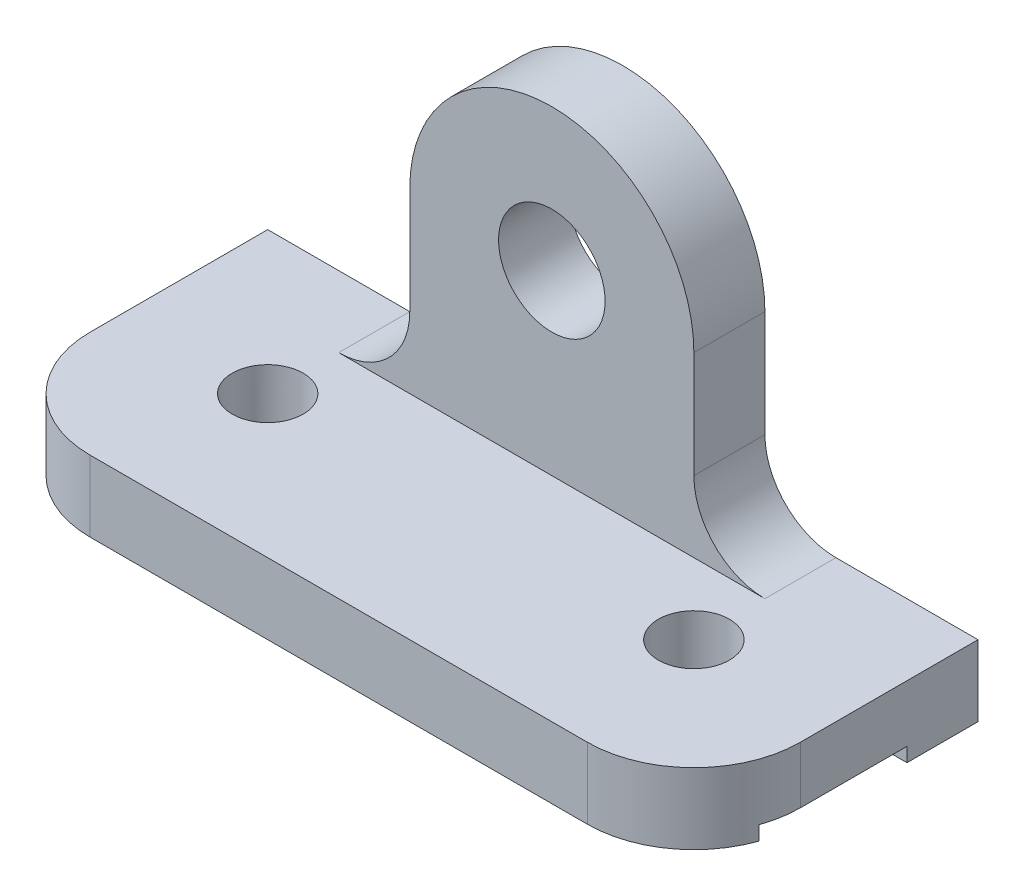
ISO-10303-21;
HEADER;
FILE_DESCRIPTION(('STEP AP214'),'2;1');
FILE_NAME('part.step','',(''),(''),'','','');
FILE_SCHEMA(('AUTOMOTIVE_DESIGN { 1 0 10303 214 1 1 1 1 }'));
ENDSEC;
DATA;
#1=APPLICATION_CONTEXT('core data for automotive mechanical design processes');
#2=APPLICATION_PROTOCOL_DEFINITION('international standard','automotive_design',2000,#1);
#3=PRODUCT_CONTEXT('',#1,'mechanical');
#4=PRODUCT('Part','Part','',(#3));
#5=PRODUCT_RELATED_PRODUCT_CATEGORY('part','',(#4));
#6=PRODUCT_DEFINITION_FORMATION('','',#4);
#7=PRODUCT_DEFINITION_CONTEXT('part definition',#1,'design');
#8=PRODUCT_DEFINITION('design','',#6,#7);
#9=PRODUCT_DEFINITION_SHAPE('','',#8);
#10=(LENGTH_UNIT() NAMED_UNIT(*) SI_UNIT(.MILLI.,.METRE.));
#11=(NAMED_UNIT(*) PLANE_ANGLE_UNIT() SI_UNIT($,.RADIAN.));
#12=(NAMED_UNIT(*) SI_UNIT($,.STERADIAN.) SOLID_ANGLE_UNIT());
#13=UNCERTAINTY_MEASURE_WITH_UNIT(LENGTH_MEASURE(1.E-05),#10,'distance_accuracy_value','');
#14=(GEOMETRIC_REPRESENTATION_CONTEXT(3) GLOBAL_UNCERTAINTY_ASSIGNED_CONTEXT((#13)) GLOBAL_UNIT_ASSIGNED_CONTEXT((#10,
#11,#12)) REPRESENTATION_CONTEXT('',''));
#15=CARTESIAN_POINT('',(0.,0.,0.));
#16=DIRECTION('',(0.,0.,1.));
#17=DIRECTION('',(1.,0.,0.));
#18=AXIS2_PLACEMENT_3D('',#15,#16,#17);
#19=CARTESIAN_POINT('',(-50.,0.,40.));
#20=DIRECTION('',(-1.,0.,0.));
#21=DIRECTION('',(0.,0.,1.));
#22=AXIS2_PLACEMENT_3D('',#19,#20,#21);
#23=PLANE('',#22);
#24=DIRECTION('',(0.,1.,0.));
#25=VECTOR('',#24,1.);
#26=CARTESIAN_POINT('',(-50.,0.,10.));
#27=LINE('',#26,#25);
#28=CARTESIAN_POINT('',(-50.,0.,10.));
#29=VERTEX_POINT('',#28);
#30=CARTESIAN_POINT('',(-50.,2.00000000000002,10.));
#31=VERTEX_POINT('',#30);
#32=EDGE_CURVE('E165',#29,#31,#27,.T.);
#33=ORIENTED_EDGE('',*,*,#32,.T.);
#34=DIRECTION('',(0.,0.,1.));
#35=VECTOR('',#34,1.);
#36=CARTESIAN_POINT('',(-50.,2.00000000000002,30.));
#37=LINE('',#36,#35);
#38=CARTESIAN_POINT('',(-50.,2.00000000000002,25.));
#39=VERTEX_POINT('',#38);
#40=EDGE_CURVE('E234',#31,#39,#37,.T.);
#41=ORIENTED_EDGE('',*,*,#40,.T.);
#42=DIRECTION('',(0.,1.,0.));
#43=VECTOR('',#42,1.);
#44=CARTESIAN_POINT('',(-50.,0.,25.));
#45=LINE('',#44,#43);
#46=CARTESIAN_POINT('',(-50.,10.,25.));
#47=VERTEX_POINT('',#46);
#48=EDGE_CURVE('E220',#39,#47,#45,.T.);
#49=ORIENTED_EDGE('',*,*,#48,.T.);
#50=DIRECTION('',(0.,0.,-1.));
#51=VECTOR('',#50,1.);
#52=CARTESIAN_POINT('',(-50.,10.,40.));
#53=LINE('',#52,#51);
#54=CARTESIAN_POINT('',(-50.,10.,0.));
#55=VERTEX_POINT('',#54);
#56=EDGE_CURVE('E184',#47,#55,#53,.T.);
#57=ORIENTED_EDGE('',*,*,#56,.T.);
#58=DIRECTION('',(0.,1.,0.));
#59=VECTOR('',#58,1.);
#60=CARTESIAN_POINT('',(-50.,0.,0.));
#61=LINE('',#60,#59);
#62=CARTESIAN_POINT('',(-50.,0.,0.));
#63=VERTEX_POINT('',#62);
#64=EDGE_CURVE('E254',#63,#55,#61,.T.);
#65=ORIENTED_EDGE('',*,*,#64,.F.);
#66=DIRECTION('',(0.,0.,-1.));
#67=VECTOR('',#66,1.);
#68=CARTESIAN_POINT('',(-50.,0.,40.));
#69=LINE('',#68,#67);
#70=EDGE_CURVE('E182',#29,#63,#69,.T.);
#71=ORIENTED_EDGE('',*,*,#70,.F.);
#72=EDGE_LOOP('',(#33,#41,#49,#57,#65,#71));
#73=FACE_BOUND('',#72,.T.);
#74=ADVANCED_FACE('F43',(#73),#23,.T.);
#75=CARTESIAN_POINT('',(0.,0.,40.));
#76=DIRECTION('',(0.,1.,0.));
#77=DIRECTION('',(-1.,0.,0.));
#78=AXIS2_PLACEMENT_3D('',#75,#76,#77);
#79=PLANE('',#78);
#80=DIRECTION('',(1.,0.,0.));
#81=VECTOR('',#80,1.);
#82=CARTESIAN_POINT('',(-50.,0.,10.));
#83=LINE('',#82,#81);
#84=CARTESIAN_POINT('',(50.,0.,10.));
#85=VERTEX_POINT('',#84);
#86=EDGE_CURVE('E156',#29,#85,#83,.T.);
#87=ORIENTED_EDGE('',*,*,#86,.F.);
#88=ORIENTED_EDGE('',*,*,#70,.T.);
#89=DIRECTION('',(1.,0.,0.));
#90=VECTOR('',#89,1.);
#91=CARTESIAN_POINT('',(0.,0.,0.));
#92=LINE('',#91,#90);
#93=CARTESIAN_POINT('',(50.,0.,0.));
#94=VERTEX_POINT('',#93);
#95=EDGE_CURVE('E178',#63,#94,#92,.T.);
#96=ORIENTED_EDGE('',*,*,#95,.T.);
#97=DIRECTION('',(0.,0.,-1.));
#98=VECTOR('',#97,1.);
#99=CARTESIAN_POINT('',(50.,0.,40.));
#100=LINE('',#99,#98);
#101=EDGE_CURVE('E172',#85,#94,#100,.T.);
#102=ORIENTED_EDGE('',*,*,#101,.F.);
#103=EDGE_LOOP('',(#87,#88,#96,#102));
#104=FACE_BOUND('',#103,.T.);
#105=ADVANCED_FACE('F180',(#104),#79,.F.);
#106=CARTESIAN_POINT('',(50.,0.,40.));
#107=DIRECTION('',(1.,0.,0.));
#108=DIRECTION('',(0.,0.,-1.));
#109=AXIS2_PLACEMENT_3D('',#106,#107,#108);
#110=PLANE('',#109);
#111=DIRECTION('',(0.,1.,0.));
#112=VECTOR('',#111,1.);
#113=CARTESIAN_POINT('',(50.,0.,10.));
#114=LINE('',#113,#112);
#115=CARTESIAN_POINT('',(50.,2.00000000000002,10.));
#116=VERTEX_POINT('',#115);
#117=EDGE_CURVE('E157',#85,#116,#114,.T.);
#118=ORIENTED_EDGE('',*,*,#117,.F.);
#119=ORIENTED_EDGE('',*,*,#101,.T.);
#120=DIRECTION('',(0.,-1.,0.));
#121=VECTOR('',#120,1.);
#122=CARTESIAN_POINT('',(50.,0.,0.));
#123=LINE('',#122,#121);
#124=CARTESIAN_POINT('',(50.,10.,0.));
#125=VERTEX_POINT('',#124);
#126=EDGE_CURVE('E257',#125,#94,#123,.T.);
#127=ORIENTED_EDGE('',*,*,#126,.F.);
#128=DIRECTION('',(0.,0.,-1.));
#129=VECTOR('',#128,1.);
#130=CARTESIAN_POINT('',(50.,10.,40.));
#131=LINE('',#130,#129);
#132=CARTESIAN_POINT('',(50.,10.,25.));
#133=VERTEX_POINT('',#132);
#134=EDGE_CURVE('E192',#133,#125,#131,.T.);
#135=ORIENTED_EDGE('',*,*,#134,.F.);
#136=DIRECTION('',(0.,-1.,0.));
#137=VECTOR('',#136,1.);
#138=CARTESIAN_POINT('',(50.,0.,25.));
#139=LINE('',#138,#137);
#140=CARTESIAN_POINT('',(50.,2.00000000000002,25.));
#141=VERTEX_POINT('',#140);
#142=EDGE_CURVE('E198',#133,#141,#139,.T.);
#143=ORIENTED_EDGE('',*,*,#142,.T.);
#144=DIRECTION('',(0.,0.,1.));
#145=VECTOR('',#144,1.);
#146=CARTESIAN_POINT('',(50.,2.00000000000002,30.));
#147=LINE('',#146,#145);
#148=EDGE_CURVE('E175',#116,#141,#147,.T.);
#149=ORIENTED_EDGE('',*,*,#148,.F.);
#150=EDGE_LOOP('',(#118,#119,#127,#135,#143,#149));
#151=FACE_BOUND('',#150,.T.);
#152=ADVANCED_FACE('F168',(#151),#110,.T.);
#153=CARTESIAN_POINT('',(0.,10.,40.));
#154=DIRECTION('',(0.,1.,0.));
#155=DIRECTION('',(-1.,0.,0.));
#156=AXIS2_PLACEMENT_3D('',#153,#154,#155);
#157=PLANE('',#156);
#158=CARTESIAN_POINT('',(30.,10.,20.));
#159=DIRECTION('',(0.,1.,0.));
#160=DIRECTION('',(-1.,0.,0.));
#161=AXIS2_PLACEMENT_3D('',#158,#159,#160);
#162=CIRCLE('',#161,5.);
#163=CARTESIAN_POINT('',(25.,10.,20.));
#164=VERTEX_POINT('',#163);
#165=EDGE_CURVE('E281',#164,#164,#162,.F.);
#166=ORIENTED_EDGE('',*,*,#165,.T.);
#167=EDGE_LOOP('',(#166));
#168=FACE_BOUND('',#167,.T.);
#169=CARTESIAN_POINT('',(-30.,10.,20.));
#170=DIRECTION('',(0.,1.,0.));
#171=DIRECTION('',(-1.,0.,0.));
#172=AXIS2_PLACEMENT_3D('',#169,#170,#171);
#173=CIRCLE('',#172,5.);
#174=CARTESIAN_POINT('',(-35.,10.,20.));
#175=VERTEX_POINT('',#174);
#176=EDGE_CURVE('E294',#175,#175,#173,.F.);
#177=ORIENTED_EDGE('',*,*,#176,.T.);
#178=EDGE_LOOP('',(#177));
#179=FACE_BOUND('',#178,.T.);
#180=DIRECTION('',(1.,0.,0.));
#181=VECTOR('',#180,1.);
#182=CARTESIAN_POINT('',(0.,10.,40.));
#183=LINE('',#182,#181);
#184=CARTESIAN_POINT('',(-35.,10.,40.));
#185=VERTEX_POINT('',#184);
#186=CARTESIAN_POINT('',(35.,10.,40.));
#187=VERTEX_POINT('',#186);
#188=EDGE_CURVE('E187',#185,#187,#183,.T.);
#189=ORIENTED_EDGE('',*,*,#188,.T.);
#190=CARTESIAN_POINT('',(35.,10.,25.));
#191=DIRECTION('',(0.,1.,0.));
#192=DIRECTION('',(-1.,0.,0.));
#193=AXIS2_PLACEMENT_3D('',#190,#191,#192);
#194=CIRCLE('',#193,15.);
#195=EDGE_CURVE('E214',#187,#133,#194,.T.);
#196=ORIENTED_EDGE('',*,*,#195,.T.);
#197=ORIENTED_EDGE('',*,*,#134,.T.);
#198=DIRECTION('',(1.,0.,0.));
#199=VECTOR('',#198,1.);
#200=CARTESIAN_POINT('',(0.,10.,0.));
#201=LINE('',#200,#199);
#202=CARTESIAN_POINT('',(30.,10.,0.));
#203=VERTEX_POINT('',#202);
#204=EDGE_CURVE('E260',#203,#125,#201,.T.);
#205=ORIENTED_EDGE('',*,*,#204,.F.);
#206=DIRECTION('',(0.,0.,-1.));
#207=VECTOR('',#206,1.);
#208=CARTESIAN_POINT('',(30.,10.,10.));
#209=LINE('',#208,#207);
#210=CARTESIAN_POINT('',(30.,10.,10.));
#211=VERTEX_POINT('',#210);
#212=EDGE_CURVE('E210',#203,#211,#209,.F.);
#213=ORIENTED_EDGE('',*,*,#212,.T.);
#214=DIRECTION('',(1.,0.,0.));
#215=VECTOR('',#214,1.);
#216=CARTESIAN_POINT('',(0.,10.,10.));
#217=LINE('',#216,#215);
#218=CARTESIAN_POINT('',(-30.,10.,10.));
#219=VERTEX_POINT('',#218);
#220=EDGE_CURVE('E283',#219,#211,#217,.T.);
#221=ORIENTED_EDGE('',*,*,#220,.F.);
#222=DIRECTION('',(0.,0.,-1.));
#223=VECTOR('',#222,1.);
#224=CARTESIAN_POINT('',(-30.,10.,40.));
#225=LINE('',#224,#223);
#226=CARTESIAN_POINT('',(-30.,10.,0.));
#227=VERTEX_POINT('',#226);
#228=EDGE_CURVE('E209',#219,#227,#225,.T.);
#229=ORIENTED_EDGE('',*,*,#228,.T.);
#230=EDGE_CURVE('E252',#55,#227,#201,.T.);
#231=ORIENTED_EDGE('',*,*,#230,.F.);
#232=ORIENTED_EDGE('',*,*,#56,.F.);
#233=CARTESIAN_POINT('',(-35.,10.,25.));
#234=DIRECTION('',(0.,1.,0.));
#235=DIRECTION('',(-1.,0.,0.));
#236=AXIS2_PLACEMENT_3D('',#233,#234,#235);
#237=CIRCLE('',#236,15.);
#238=EDGE_CURVE('E213',#47,#185,#237,.T.);
#239=ORIENTED_EDGE('',*,*,#238,.T.);
#240=EDGE_LOOP('',(#189,#196,#197,#205,#213,#221,#229,#231,#232,#239));
#241=FACE_BOUND('',#240,.T.);
#242=ADVANCED_FACE('F249',(#168,#179,#241),#157,.T.);
#243=CARTESIAN_POINT('',(-35.,0.,25.));
#244=DIRECTION('',(0.,1.,0.));
#245=DIRECTION('',(-1.,0.,0.));
#246=AXIS2_PLACEMENT_3D('',#243,#244,#245);
#247=CIRCLE('',#246,15.);
#248=CARTESIAN_POINT('',(-35.,0.,40.));
#249=VERTEX_POINT('',#248);
#250=CARTESIAN_POINT('',(-49.142135623731,0.,30.));
#251=VERTEX_POINT('',#250);
#252=EDGE_CURVE('E196',#249,#251,#247,.F.);
#253=ORIENTED_EDGE('',*,*,#252,.T.);
#254=DIRECTION('',(1.,0.,0.));
#255=VECTOR('',#254,1.);
#256=CARTESIAN_POINT('',(-50.,0.,30.));
#257=LINE('',#256,#255);
#258=CARTESIAN_POINT('',(49.142135623731,0.,30.));
#259=VERTEX_POINT('',#258);
#260=EDGE_CURVE('E170',#251,#259,#257,.T.);
#261=ORIENTED_EDGE('',*,*,#260,.T.);
#262=CARTESIAN_POINT('',(35.,0.,25.));
#263=DIRECTION('',(0.,1.,0.));
#264=DIRECTION('',(-1.,0.,0.));
#265=AXIS2_PLACEMENT_3D('',#262,#263,#264);
#266=CIRCLE('',#265,15.);
#267=CARTESIAN_POINT('',(35.,0.,40.));
#268=VERTEX_POINT('',#267);
#269=EDGE_CURVE('E203',#259,#268,#266,.F.);
#270=ORIENTED_EDGE('',*,*,#269,.T.);
#271=DIRECTION('',(1.,0.,0.));
#272=VECTOR('',#271,1.);
#273=CARTESIAN_POINT('',(0.,0.,40.));
#274=LINE('',#273,#272);
#275=EDGE_CURVE('E185',#249,#268,#274,.T.);
#276=ORIENTED_EDGE('',*,*,#275,.F.);
#277=EDGE_LOOP('',(#253,#261,#270,#276));
#278=FACE_BOUND('',#277,.T.);
#279=ADVANCED_FACE('F330',(#278),#79,.F.);
#280=CARTESIAN_POINT('',(0.,0.,40.));
#281=DIRECTION('',(0.,0.,1.));
#282=DIRECTION('',(1.,0.,0.));
#283=AXIS2_PLACEMENT_3D('',#280,#281,#282);
#284=PLANE('',#283);
#285=ORIENTED_EDGE('',*,*,#275,.T.);
#286=DIRECTION('',(0.,-1.,0.));
#287=VECTOR('',#286,1.);
#288=CARTESIAN_POINT('',(35.,0.,40.));
#289=LINE('',#288,#287);
#290=EDGE_CURVE('E202',#268,#187,#289,.F.);
#291=ORIENTED_EDGE('',*,*,#290,.T.);
#292=ORIENTED_EDGE('',*,*,#188,.F.);
#293=DIRECTION('',(0.,1.,0.));
#294=VECTOR('',#293,1.);
#295=CARTESIAN_POINT('',(-35.,0.,40.));
#296=LINE('',#295,#294);
#297=EDGE_CURVE('E201',#185,#249,#296,.F.);
#298=ORIENTED_EDGE('',*,*,#297,.T.);
#299=EDGE_LOOP('',(#285,#291,#292,#298));
#300=FACE_BOUND('',#299,.T.);
#301=ADVANCED_FACE('F322',(#300),#284,.T.);
#302=CARTESIAN_POINT('',(0.,0.,0.));
#303=DIRECTION('',(0.,0.,1.));
#304=DIRECTION('',(1.,0.,0.));
#305=AXIS2_PLACEMENT_3D('',#302,#303,#304);
#306=PLANE('',#305);
#307=ORIENTED_EDGE('',*,*,#126,.T.);
#308=ORIENTED_EDGE('',*,*,#95,.F.);
#309=ORIENTED_EDGE('',*,*,#64,.T.);
#310=ORIENTED_EDGE('',*,*,#230,.T.);
#311=CARTESIAN_POINT('',(-30.,20.,0.));
#312=DIRECTION('',(0.,0.,1.));
#313=DIRECTION('',(1.,0.,0.));
#314=AXIS2_PLACEMENT_3D('',#311,#312,#313);
#315=CIRCLE('',#314,10.);
#316=CARTESIAN_POINT('',(-20.,20.,0.));
#317=VERTEX_POINT('',#316);
#318=EDGE_CURVE('E221',#227,#317,#315,.T.);
#319=ORIENTED_EDGE('',*,*,#318,.T.);
#320=DIRECTION('',(0.,-1.,0.));
#321=VECTOR('',#320,1.);
#322=CARTESIAN_POINT('',(-20.,0.,0.));
#323=LINE('',#322,#321);
#324=CARTESIAN_POINT('',(-20.,35.,0.));
#325=VERTEX_POINT('',#324);
#326=EDGE_CURVE('E272',#325,#317,#323,.T.);
#327=ORIENTED_EDGE('',*,*,#326,.F.);
#328=CARTESIAN_POINT('',(0.,35.,0.));
#329=DIRECTION('',(0.,0.,1.));
#330=DIRECTION('',(1.,0.,0.));
#331=AXIS2_PLACEMENT_3D('',#328,#329,#330);
#332=CIRCLE('',#331,20.);
#333=CARTESIAN_POINT('',(20.,35.,0.));
#334=VERTEX_POINT('',#333);
#335=EDGE_CURVE('E277',#334,#325,#332,.T.);
#336=ORIENTED_EDGE('',*,*,#335,.F.);
#337=DIRECTION('',(0.,-1.,0.));
#338=VECTOR('',#337,1.);
#339=CARTESIAN_POINT('',(20.,0.,0.));
#340=LINE('',#339,#338);
#341=CARTESIAN_POINT('',(20.,20.,0.));
#342=VERTEX_POINT('',#341);
#343=EDGE_CURVE('E279',#334,#342,#340,.T.);
#344=ORIENTED_EDGE('',*,*,#343,.T.);
#345=CARTESIAN_POINT('',(30.,20.,0.));
#346=DIRECTION('',(0.,0.,1.));
#347=DIRECTION('',(1.,0.,0.));
#348=AXIS2_PLACEMENT_3D('',#345,#346,#347);
#349=CIRCLE('',#348,10.);
#350=EDGE_CURVE('E228',#342,#203,#349,.T.);
#351=ORIENTED_EDGE('',*,*,#350,.T.);
#352=ORIENTED_EDGE('',*,*,#204,.T.);
#353=EDGE_LOOP('',(#307,#308,#309,#310,#319,#327,#336,#344,#351,#352));
#354=FACE_BOUND('',#353,.T.);
#355=CARTESIAN_POINT('',(0.,35.,0.));
#356=DIRECTION('',(0.,0.,1.));
#357=DIRECTION('',(1.,0.,0.));
#358=AXIS2_PLACEMENT_3D('',#355,#356,#357);
#359=CIRCLE('',#358,7.5);
#360=CARTESIAN_POINT('',(7.5,35.,0.));
#361=VERTEX_POINT('',#360);
#362=EDGE_CURVE('E267',#361,#361,#359,.T.);
#363=ORIENTED_EDGE('',*,*,#362,.T.);
#364=EDGE_LOOP('',(#363));
#365=FACE_BOUND('',#364,.T.);
#366=ADVANCED_FACE('F376',(#354,#365),#306,.F.);
#367=CARTESIAN_POINT('',(20.,0.,10.));
#368=DIRECTION('',(1.,0.,0.));
#369=DIRECTION('',(0.,0.,-1.));
#370=AXIS2_PLACEMENT_3D('',#367,#368,#369);
#371=PLANE('',#370);
#372=DIRECTION('',(0.,-1.,0.));
#373=VECTOR('',#372,1.);
#374=CARTESIAN_POINT('',(20.,0.,10.));
#375=LINE('',#374,#373);
#376=CARTESIAN_POINT('',(20.,35.,10.));
#377=VERTEX_POINT('',#376);
#378=CARTESIAN_POINT('',(20.,20.,10.));
#379=VERTEX_POINT('',#378);
#380=EDGE_CURVE('E275',#377,#379,#375,.T.);
#381=ORIENTED_EDGE('',*,*,#380,.T.);
#382=DIRECTION('',(0.,0.,-1.));
#383=VECTOR('',#382,1.);
#384=CARTESIAN_POINT('',(20.,20.,0.));
#385=LINE('',#384,#383);
#386=EDGE_CURVE('E222',#379,#342,#385,.T.);
#387=ORIENTED_EDGE('',*,*,#386,.T.);
#388=ORIENTED_EDGE('',*,*,#343,.F.);
#389=DIRECTION('',(0.,0.,-1.));
#390=VECTOR('',#389,1.);
#391=CARTESIAN_POINT('',(20.,35.,10.));
#392=LINE('',#391,#390);
#393=EDGE_CURVE('E261',#377,#334,#392,.T.);
#394=ORIENTED_EDGE('',*,*,#393,.F.);
#395=EDGE_LOOP('',(#381,#387,#388,#394));
#396=FACE_BOUND('',#395,.T.);
#397=ADVANCED_FACE('F381',(#396),#371,.T.);
#398=CARTESIAN_POINT('',(0.,35.,10.));
#399=DIRECTION('',(0.,0.,-1.));
#400=DIRECTION('',(-1.,0.,0.));
#401=AXIS2_PLACEMENT_3D('',#398,#399,#400);
#402=CYLINDRICAL_SURFACE('',#401,20.);
#403=ORIENTED_EDGE('',*,*,#335,.T.);
#404=DIRECTION('',(0.,0.,-1.));
#405=VECTOR('',#404,1.);
#406=CARTESIAN_POINT('',(-20.,35.,10.));
#407=LINE('',#406,#405);
#408=CARTESIAN_POINT('',(-20.,35.,10.));
#409=VERTEX_POINT('',#408);
#410=EDGE_CURVE('E264',#409,#325,#407,.T.);
#411=ORIENTED_EDGE('',*,*,#410,.F.);
#412=CARTESIAN_POINT('',(0.,35.,10.));
#413=DIRECTION('',(0.,0.,1.));
#414=DIRECTION('',(1.,0.,0.));
#415=AXIS2_PLACEMENT_3D('',#412,#413,#414);
#416=CIRCLE('',#415,20.);
#417=EDGE_CURVE('E288',#377,#409,#416,.T.);
#418=ORIENTED_EDGE('',*,*,#417,.F.);
#419=ORIENTED_EDGE('',*,*,#393,.T.);
#420=EDGE_LOOP('',(#403,#411,#418,#419));
#421=FACE_BOUND('',#420,.T.);
#422=ADVANCED_FACE('F382',(#421),#402,.T.);
#423=CARTESIAN_POINT('',(-20.,0.,10.));
#424=DIRECTION('',(1.,0.,0.));
#425=DIRECTION('',(0.,0.,-1.));
#426=AXIS2_PLACEMENT_3D('',#423,#424,#425);
#427=PLANE('',#426);
#428=ORIENTED_EDGE('',*,*,#326,.T.);
#429=DIRECTION('',(0.,0.,-1.));
#430=VECTOR('',#429,1.);
#431=CARTESIAN_POINT('',(-20.,20.,10.));
#432=LINE('',#431,#430);
#433=CARTESIAN_POINT('',(-20.,20.,10.));
#434=VERTEX_POINT('',#433);
#435=EDGE_CURVE('E218',#317,#434,#432,.F.);
#436=ORIENTED_EDGE('',*,*,#435,.T.);
#437=DIRECTION('',(0.,-1.,0.));
#438=VECTOR('',#437,1.);
#439=CARTESIAN_POINT('',(-20.,0.,10.));
#440=LINE('',#439,#438);
#441=EDGE_CURVE('E286',#409,#434,#440,.T.);
#442=ORIENTED_EDGE('',*,*,#441,.F.);
#443=ORIENTED_EDGE('',*,*,#410,.T.);
#444=EDGE_LOOP('',(#428,#436,#442,#443));
#445=FACE_BOUND('',#444,.T.);
#446=ADVANCED_FACE('F373',(#445),#427,.F.);
#447=CARTESIAN_POINT('',(0.,35.,10.));
#448=DIRECTION('',(0.,0.,-1.));
#449=DIRECTION('',(-1.,0.,0.));
#450=AXIS2_PLACEMENT_3D('',#447,#448,#449);
#451=CYLINDRICAL_SURFACE('',#450,7.5);
#452=CARTESIAN_POINT('',(0.,35.,10.));
#453=DIRECTION('',(0.,0.,1.));
#454=DIRECTION('',(1.,0.,0.));
#455=AXIS2_PLACEMENT_3D('',#452,#453,#454);
#456=CIRCLE('',#455,7.5);
#457=CARTESIAN_POINT('',(7.5,35.,10.));
#458=VERTEX_POINT('',#457);
#459=EDGE_CURVE('E268',#458,#458,#456,.T.);
#460=ORIENTED_EDGE('',*,*,#459,.T.);
#461=EDGE_LOOP('',(#460));
#462=FACE_BOUND('',#461,.T.);
#463=ORIENTED_EDGE('',*,*,#362,.F.);
#464=EDGE_LOOP('',(#463));
#465=FACE_BOUND('',#464,.T.);
#466=ADVANCED_FACE('F388',(#462,#465),#451,.F.);
#467=CARTESIAN_POINT('',(0.,0.,10.));
#468=DIRECTION('',(0.,0.,1.));
#469=DIRECTION('',(1.,0.,0.));
#470=AXIS2_PLACEMENT_3D('',#467,#468,#469);
#471=PLANE('',#470);
#472=ORIENTED_EDGE('',*,*,#380,.F.);
#473=ORIENTED_EDGE('',*,*,#417,.T.);
#474=ORIENTED_EDGE('',*,*,#441,.T.);
#475=CARTESIAN_POINT('',(-30.,20.,10.));
#476=DIRECTION('',(0.,0.,1.));
#477=DIRECTION('',(1.,0.,0.));
#478=AXIS2_PLACEMENT_3D('',#475,#476,#477);
#479=CIRCLE('',#478,10.);
#480=EDGE_CURVE('E226',#434,#219,#479,.F.);
#481=ORIENTED_EDGE('',*,*,#480,.T.);
#482=ORIENTED_EDGE('',*,*,#220,.T.);
#483=CARTESIAN_POINT('',(30.,20.,10.));
#484=DIRECTION('',(0.,0.,1.));
#485=DIRECTION('',(1.,0.,0.));
#486=AXIS2_PLACEMENT_3D('',#483,#484,#485);
#487=CIRCLE('',#486,10.);
#488=EDGE_CURVE('E65',#211,#379,#487,.F.);
#489=ORIENTED_EDGE('',*,*,#488,.T.);
#490=EDGE_LOOP('',(#472,#473,#474,#481,#482,#489));
#491=FACE_BOUND('',#490,.T.);
#492=ORIENTED_EDGE('',*,*,#459,.F.);
#493=EDGE_LOOP('',(#492));
#494=FACE_BOUND('',#493,.T.);
#495=ADVANCED_FACE('F370',(#491,#494),#471,.T.);
#496=CARTESIAN_POINT('',(-30.,55.,20.));
#497=DIRECTION('',(0.,-1.,0.));
#498=DIRECTION('',(1.,0.,0.));
#499=AXIS2_PLACEMENT_3D('',#496,#497,#498);
#500=CYLINDRICAL_SURFACE('',#499,5.);
#501=CARTESIAN_POINT('',(-30.,2.00000000000002,20.));
#502=DIRECTION('',(0.,1.,0.));
#503=DIRECTION('',(0.,0.,1.));
#504=AXIS2_PLACEMENT_3D('',#501,#502,#503);
#505=CIRCLE('',#504,5.);
#506=CARTESIAN_POINT('',(-30.,2.00000000000002,25.));
#507=VERTEX_POINT('',#506);
#508=EDGE_CURVE('E298',#507,#507,#505,.T.);
#509=ORIENTED_EDGE('',*,*,#508,.F.);
#510=EDGE_LOOP('',(#509));
#511=FACE_BOUND('',#510,.T.);
#512=ORIENTED_EDGE('',*,*,#176,.F.);
#513=EDGE_LOOP('',(#512));
#514=FACE_BOUND('',#513,.T.);
#515=ADVANCED_FACE('F416',(#511,#514),#500,.F.);
#516=CARTESIAN_POINT('',(30.,55.,20.));
#517=DIRECTION('',(0.,-1.,0.));
#518=DIRECTION('',(1.,0.,0.));
#519=AXIS2_PLACEMENT_3D('',#516,#517,#518);
#520=CYLINDRICAL_SURFACE('',#519,5.);
#521=CARTESIAN_POINT('',(30.,2.00000000000002,20.));
#522=DIRECTION('',(0.,1.,0.));
#523=DIRECTION('',(0.,0.,1.));
#524=AXIS2_PLACEMENT_3D('',#521,#522,#523);
#525=CIRCLE('',#524,5.);
#526=CARTESIAN_POINT('',(30.,2.00000000000002,25.));
#527=VERTEX_POINT('',#526);
#528=EDGE_CURVE('E305',#527,#527,#525,.T.);
#529=ORIENTED_EDGE('',*,*,#528,.F.);
#530=EDGE_LOOP('',(#529));
#531=FACE_BOUND('',#530,.T.);
#532=ORIENTED_EDGE('',*,*,#165,.F.);
#533=EDGE_LOOP('',(#532));
#534=FACE_BOUND('',#533,.T.);
#535=ADVANCED_FACE('F357',(#531,#534),#520,.F.);
#536=CARTESIAN_POINT('',(35.,0.,25.));
#537=DIRECTION('',(0.,-1.,0.));
#538=DIRECTION('',(0.,0.,-1.));
#539=AXIS2_PLACEMENT_3D('',#536,#537,#538);
#540=CYLINDRICAL_SURFACE('',#539,15.);
#541=DIRECTION('',(0.,-1.,0.));
#542=VECTOR('',#541,1.);
#543=CARTESIAN_POINT('',(49.142135623731,0.,30.));
#544=LINE('',#543,#542);
#545=CARTESIAN_POINT('',(49.142135623731,2.00000000000002,30.));
#546=VERTEX_POINT('',#545);
#547=EDGE_CURVE('E297',#546,#259,#544,.T.);
#548=ORIENTED_EDGE('',*,*,#547,.F.);
#549=CARTESIAN_POINT('',(35.,2.00000000000002,25.));
#550=DIRECTION('',(0.,1.,0.));
#551=DIRECTION('',(0.,0.,1.));
#552=AXIS2_PLACEMENT_3D('',#549,#550,#551);
#553=CIRCLE('',#552,15.);
#554=EDGE_CURVE('E304',#141,#546,#553,.F.);
#555=ORIENTED_EDGE('',*,*,#554,.F.);
#556=ORIENTED_EDGE('',*,*,#142,.F.);
#557=ORIENTED_EDGE('',*,*,#195,.F.);
#558=ORIENTED_EDGE('',*,*,#290,.F.);
#559=ORIENTED_EDGE('',*,*,#269,.F.);
#560=EDGE_LOOP('',(#548,#555,#556,#557,#558,#559));
#561=FACE_BOUND('',#560,.T.);
#562=ADVANCED_FACE('F316',(#561),#540,.T.);
#563=CARTESIAN_POINT('',(-35.,0.,25.));
#564=DIRECTION('',(0.,1.,0.));
#565=DIRECTION('',(0.,0.,1.));
#566=AXIS2_PLACEMENT_3D('',#563,#564,#565);
#567=CYLINDRICAL_SURFACE('',#566,15.);
#568=DIRECTION('',(0.,1.,0.));
#569=VECTOR('',#568,1.);
#570=CARTESIAN_POINT('',(-49.142135623731,0.,30.));
#571=LINE('',#570,#569);
#572=CARTESIAN_POINT('',(-49.142135623731,2.00000000000002,30.));
#573=VERTEX_POINT('',#572);
#574=EDGE_CURVE('E12',#251,#573,#571,.T.);
#575=ORIENTED_EDGE('',*,*,#574,.F.);
#576=ORIENTED_EDGE('',*,*,#252,.F.);
#577=ORIENTED_EDGE('',*,*,#297,.F.);
#578=ORIENTED_EDGE('',*,*,#238,.F.);
#579=ORIENTED_EDGE('',*,*,#48,.F.);
#580=CARTESIAN_POINT('',(-35.,2.00000000000002,25.));
#581=DIRECTION('',(0.,1.,0.));
#582=DIRECTION('',(0.,0.,1.));
#583=AXIS2_PLACEMENT_3D('',#580,#581,#582);
#584=CIRCLE('',#583,15.);
#585=EDGE_CURVE('E51',#573,#39,#584,.F.);
#586=ORIENTED_EDGE('',*,*,#585,.F.);
#587=EDGE_LOOP('',(#575,#576,#577,#578,#579,#586));
#588=FACE_BOUND('',#587,.T.);
#589=ADVANCED_FACE('F242',(#588),#567,.T.);
#590=CARTESIAN_POINT('',(-30.,20.,40.));
#591=DIRECTION('',(0.,0.,-1.));
#592=DIRECTION('',(-1.,0.,0.));
#593=AXIS2_PLACEMENT_3D('',#590,#591,#592);
#594=CYLINDRICAL_SURFACE('',#593,10.);
#595=ORIENTED_EDGE('',*,*,#480,.F.);
#596=ORIENTED_EDGE('',*,*,#435,.F.);
#597=ORIENTED_EDGE('',*,*,#318,.F.);
#598=ORIENTED_EDGE('',*,*,#228,.F.);
#599=EDGE_LOOP('',(#595,#596,#597,#598));
#600=FACE_BOUND('',#599,.T.);
#601=ADVANCED_FACE('F338',(#600),#594,.F.);
#602=CARTESIAN_POINT('',(30.,20.,10.));
#603=DIRECTION('',(0.,0.,1.));
#604=DIRECTION('',(1.,0.,0.));
#605=AXIS2_PLACEMENT_3D('',#602,#603,#604);
#606=CYLINDRICAL_SURFACE('',#605,10.);
#607=ORIENTED_EDGE('',*,*,#488,.F.);
#608=ORIENTED_EDGE('',*,*,#212,.F.);
#609=ORIENTED_EDGE('',*,*,#350,.F.);
#610=ORIENTED_EDGE('',*,*,#386,.F.);
#611=EDGE_LOOP('',(#607,#608,#609,#610));
#612=FACE_BOUND('',#611,.T.);
#613=ADVANCED_FACE('F44',(#612),#606,.F.);
#614=CARTESIAN_POINT('',(-50.,0.,30.));
#615=DIRECTION('',(0.,0.,1.));
#616=DIRECTION('',(1.,0.,0.));
#617=AXIS2_PLACEMENT_3D('',#614,#615,#616);
#618=PLANE('',#617);
#619=ORIENTED_EDGE('',*,*,#547,.T.);
#620=ORIENTED_EDGE('',*,*,#260,.F.);
#621=ORIENTED_EDGE('',*,*,#574,.T.);
#622=DIRECTION('',(1.,0.,0.));
#623=VECTOR('',#622,1.);
#624=CARTESIAN_POINT('',(-50.,2.00000000000002,30.));
#625=LINE('',#624,#623);
#626=EDGE_CURVE('E59',#573,#546,#625,.T.);
#627=ORIENTED_EDGE('',*,*,#626,.T.);
#628=EDGE_LOOP('',(#619,#620,#621,#627));
#629=FACE_BOUND('',#628,.T.);
#630=ADVANCED_FACE('F328',(#629),#618,.F.);
#631=CARTESIAN_POINT('',(-50.,2.00000000000002,30.));
#632=DIRECTION('',(0.,1.,0.));
#633=DIRECTION('',(0.,0.,1.));
#634=AXIS2_PLACEMENT_3D('',#631,#632,#633);
#635=PLANE('',#634);
#636=ORIENTED_EDGE('',*,*,#508,.T.);
#637=EDGE_LOOP('',(#636));
#638=FACE_BOUND('',#637,.T.);
#639=ORIENTED_EDGE('',*,*,#528,.T.);
#640=EDGE_LOOP('',(#639));
#641=FACE_BOUND('',#640,.T.);
#642=ORIENTED_EDGE('',*,*,#554,.T.);
#643=ORIENTED_EDGE('',*,*,#626,.F.);
#644=ORIENTED_EDGE('',*,*,#585,.T.);
#645=ORIENTED_EDGE('',*,*,#40,.F.);
#646=DIRECTION('',(1.,0.,0.));
#647=VECTOR('',#646,1.);
#648=CARTESIAN_POINT('',(-50.,2.00000000000002,10.));
#649=LINE('',#648,#647);
#650=EDGE_CURVE('E167',#31,#116,#649,.T.);
#651=ORIENTED_EDGE('',*,*,#650,.T.);
#652=ORIENTED_EDGE('',*,*,#148,.T.);
#653=EDGE_LOOP('',(#642,#643,#644,#645,#651,#652));
#654=FACE_BOUND('',#653,.T.);
#655=ADVANCED_FACE('F233',(#638,#641,#654),#635,.F.);
#656=CARTESIAN_POINT('',(-50.,0.,10.));
#657=DIRECTION('',(0.,0.,-1.));
#658=DIRECTION('',(0.,1.,0.));
#659=AXIS2_PLACEMENT_3D('',#656,#657,#658);
#660=PLANE('',#659);
#661=ORIENTED_EDGE('',*,*,#650,.F.);
#662=ORIENTED_EDGE('',*,*,#32,.F.);
#663=ORIENTED_EDGE('',*,*,#86,.T.);
#664=ORIENTED_EDGE('',*,*,#117,.T.);
#665=EDGE_LOOP('',(#661,#662,#663,#664));
#666=FACE_BOUND('',#665,.T.);
#667=ADVANCED_FACE('F158',(#666),#660,.F.);
#668=CLOSED_SHELL('',(#74,#105,#152,#242,#279,#301,#366,#397,#422,#446,#466,#495,#515,#535,#562,
#589,#601,#613,#630,#655,#667));
#669=MANIFOLD_SOLID_BREP('B2',#668);
#670=ADVANCED_BREP_SHAPE_REPRESENTATION('',(#18,#669),#14);
#671=SHAPE_DEFINITION_REPRESENTATION(#9,#670);
ENDSEC;
END-ISO-10303-21;
